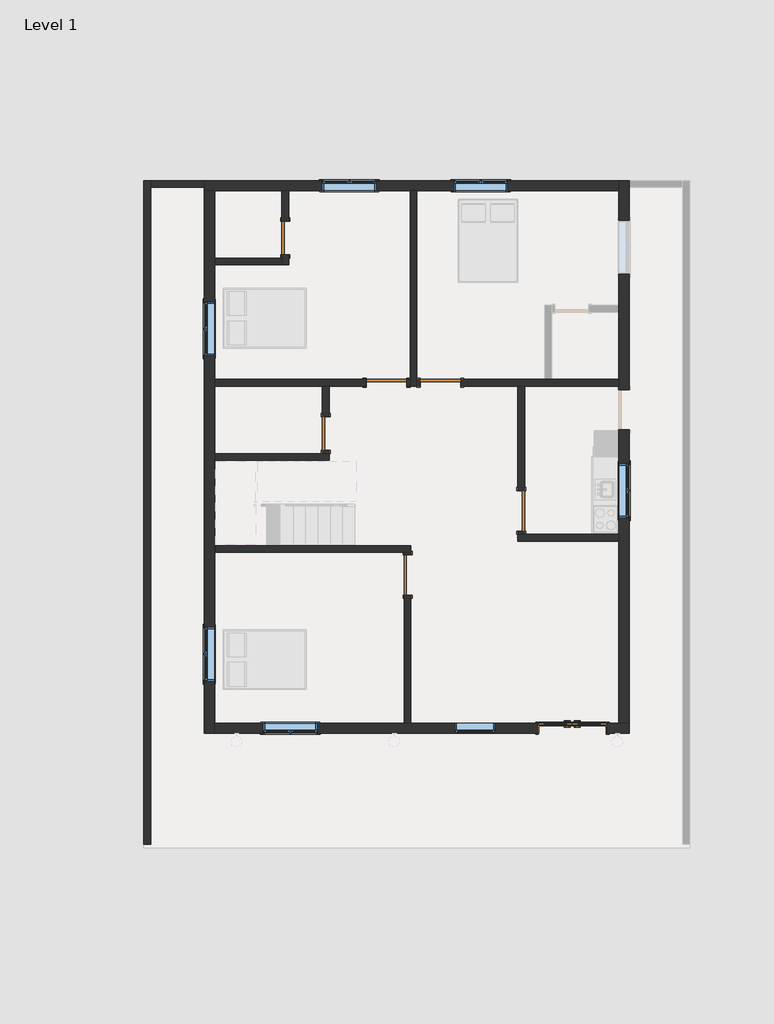
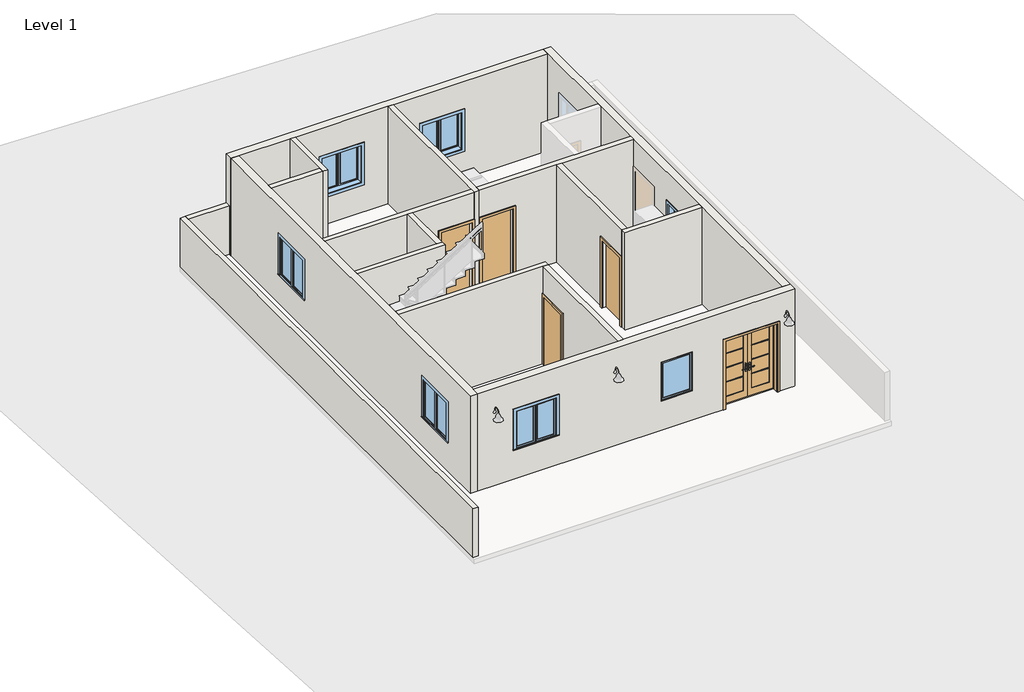
# One storey, part 1 of 2: 17 walls, 7 doors, 7 windows.
"""IFC4 building model written with IfcOpenShell, lengths in millimetres."""

from ifc_helpers import new_model, si_unit, frame, origin, origin_with_axes, place, context, project, spatial, polyline, outline, extrude, faceted_brep, transform, mapped, element, save
from components import door_014e9f54, single_flush_2_5_e2b13fe9, door_16372e1c, door_686f89d2, window_8af0dca1, window_c1f32544

model = new_model("IFC4")

# Units and contexts
model_context = context("Model", 3, world=origin())
ifc_project = project(units=[si_unit("LENGTHUNIT", "METRE", prefix="MILLI")], contexts=[model_context])

# Site, building, storey
site = spatial("IfcSite", under=ifc_project)
building = spatial("IfcBuilding", under=site)
storey = spatial("IfcBuildingStorey", under=building, Name="Level 1", Elevation=0.0)

# Doors
placement = place(None, origin())
door_shape = door_014e9f54(model_context)
element("IfcDoor", 1, ObjectType="Door-Exterior-Double-Full Glass-Wood_Clad : 60\" x 84\"", at=placement, inside=storey, context=model_context, shape_type="MappedRepresentation", body=[
    mapped(door_shape, transform((605.0352982, -4712.4924812, 0.0), x_axis=(1.0, 0.0, 0.0), y_axis=(0.0, 1.0, 0.0), z_axis=(0.0, 0.0, 1.0))),
])
single_flush_2_5_shape = single_flush_2_5_e2b13fe9(model_context)
element("IfcDoor", 2, ObjectType="Single-Flush : 2.5'", at=placement, inside=storey, context=model_context, shape_type="MappedRepresentation", body=[
    mapped(single_flush_2_5_shape, transform((-5884.6647018, 6371.4325188, 0.0), x_axis=(0.0, -1.0, 0.0), y_axis=(1.0, 0.0, 0.0), z_axis=(0.0, 0.0, 1.0))),
])
element("IfcDoor", 3, ObjectType="Single-Flush : 2.5'", at=placement, inside=storey, context=model_context, shape_type="MappedRepresentation", body=[
    mapped(single_flush_2_5_shape, transform((-4970.2647018, 1951.8325188, 0.0), x_axis=(0.0, -1.0, 0.0), y_axis=(1.0, 0.0, 0.0), z_axis=(0.0, 0.0, 1.0))),
])
door_2_shape = door_16372e1c(model_context)
element("IfcDoor", 4, ObjectType="Single-Flush : 36\" x 84\"", at=placement, inside=storey, context=model_context, shape_type="MappedRepresentation", body=[
    mapped(door_2_shape, transform((-3119.9591614, -1248.0450563, 0.0), x_axis=(0.0, 1.0, 0.0), y_axis=(-1.0, 0.0, 0.0), z_axis=(0.0, 0.0, 1.0))),
])
element("IfcDoor", 5, ObjectType="Single-Flush : 36\" x 84\"", at=placement, inside=storey, context=model_context, shape_type="MappedRepresentation", body=[
    mapped(door_2_shape, transform((-3598.6647018, 3094.8325188, 0.0), x_axis=(1.0, 0.0, 0.0), y_axis=(0.0, 1.0, 0.0), z_axis=(0.0, 0.0, 1.0))),
])
element("IfcDoor", 6, ObjectType="Single-Flush : 36\" x 84\"", at=placement, inside=storey, context=model_context, shape_type="MappedRepresentation", body=[
    mapped(door_2_shape, transform((-550.6647018, 199.2325188, 0.0), x_axis=(0.0, -1.0, 0.0), y_axis=(1.0, 0.0, 0.0), z_axis=(0.0, 0.0, 1.0))),
])
door_3_shape = door_686f89d2(model_context)
element("IfcDoor", 7, ObjectType="Single-Flush : 36\" x 84\"", at=placement, inside=storey, context=model_context, shape_type="MappedRepresentation", body=[
    mapped(door_3_shape, transform((-2379.4647018, 3094.8325188, 0.0), x_axis=(-1.0, 0.0, 0.0), y_axis=(0.0, -1.0, 0.0), z_axis=(0.0, 0.0, 1.0))),
])

# Walls
element("IfcWall", 8, ObjectType="6\"", at=placement, inside=storey, context=model_context, shape_type="Brep", body=[
    faceted_brep([(-8932.6647018, -7344.5674812, 0.0), (-8932.6647018, 7514.4325188, 0.0), (-8932.6647018, 7666.8325188, 0.0), (-8932.6647018, 7666.8325188, 1524.0), (-8932.6647018, 7514.4325188, 1524.0), (-8932.6647018, -7344.5674812, 1524.0), (-9085.0647018, -7344.5674812, 0.0), (-9085.0647018, -7344.5674812, 1524.0), (-9085.0647018, 7666.8325188, 1524.0), (-9085.0647018, 7666.8325188, 0.0)], [[[0, 1, 2, 3, 4, 5]], [[6, 7, 8, 9]], [[2, 1, 0, 6, 9]], [[5, 4, 3, 8, 7]], [[0, 5, 7, 6]], [[3, 2, 9, 8]]]),
])
element("IfcWall", 9, ObjectType="6\"", at=placement, inside=storey, context=model_context, shape_type="Brep", body=[
    faceted_brep([(-3065.2647018, 7438.2325188, 0.0), (-3065.2647018, 3171.0325188, 0.0), (-3065.2647018, 3018.6325188, 0.0), (-3065.2647018, 3018.6325188, 3048.0), (-3065.2647018, 3171.0325188, 3048.0), (-3065.2647018, 7438.2325188, 3048.0), (-2912.8647018, 7438.2325188, 0.0), (-2912.8647018, 7438.2325188, 3048.0), (-2912.8647018, 3171.0325188, 3048.0), (-2912.8647018, 3018.6325188, 3048.0), (-2912.8647018, 3018.6325188, 0.0), (-2912.8647018, 3171.0325188, 0.0)], [[[0, 1, 2, 3, 4, 5]], [[6, 7, 8, 9, 10, 11]], [[2, 1, 0, 6, 11, 10]], [[5, 4, 3, 9, 8, 7]], [[0, 5, 7, 6]], [[3, 2, 10, 9]]]),
])
element("IfcWall", 10, ObjectType="6\"", at=placement, inside=storey, context=model_context, shape_type="Brep", body=[
    faceted_brep([(-3065.2647018, 3171.0325188, 0.0), (-3141.4647018, 3171.0325188, 0.0), (-3141.4647018, 3171.0325188, 2133.6), (-4055.8647018, 3171.0325188, 2133.6), (-4055.8647018, 3171.0325188, 0.0), (-7484.8647018, 3171.0325188, 0.0), (-7484.8647018, 3171.0325188, 3048.0), (-3065.2647018, 3171.0325188, 3048.0), (-3141.4647018, 3018.6325188, 2133.6), (-3141.4647018, 3018.6325188, 0.0), (-3065.2647018, 3018.6325188, 0.0), (-3065.2647018, 3018.6325188, 3048.0), (-4894.0647018, 3018.6325188, 3048.0), (-5046.4647018, 3018.6325188, 3048.0), (-7484.8647018, 3018.6325188, 3048.0), (-7484.8647018, 3018.6325188, 0.0), (-5046.4647018, 3018.6325188, 0.0), (-4894.0647018, 3018.6325188, 0.0), (-4055.8647018, 3018.6325188, 0.0), (-4055.8647018, 3018.6325188, 2133.6)], [[[0, 1, 2, 3, 4, 5, 6, 7]], [[8, 9, 10, 11, 12, 13, 14, 15, 16, 17, 18, 19]], [[10, 9, 1, 0]], [[18, 17, 16, 15, 5, 4]], [[7, 6, 14, 13, 12, 11]], [[0, 7, 11, 10]], [[6, 5, 15, 14]], [[2, 1, 9, 8]], [[3, 2, 8, 19]], [[4, 3, 19, 18]]]),
])
element("IfcWall", 11, ObjectType="6\"", at=placement, inside=storey, context=model_context, shape_type="Brep", body=[
    faceted_brep([(-2912.8647018, 3018.6325188, 0.0), (-2836.6647018, 3018.6325188, 0.0), (-2836.6647018, 3018.6325188, 2133.6), (-1922.2647018, 3018.6325188, 2133.6), (-1922.2647018, 3018.6325188, 0.0), (-626.8647018, 3018.6325188, 0.0), (-474.4647018, 3018.6325188, 0.0), (1659.1352982, 3018.6325188, 0.0), (1659.1352982, 3018.6325188, 3048.0), (-474.4647018, 3018.6325188, 3048.0), (-626.8647018, 3018.6325188, 3048.0), (-2912.8647018, 3018.6325188, 3048.0), (-2836.6647018, 3171.0325188, 2133.6), (-2836.6647018, 3171.0325188, 0.0), (-2912.8647018, 3171.0325188, 0.0), (-2912.8647018, 3171.0325188, 3048.0), (-17.2647018, 3171.0325188, 3048.0), (135.1352982, 3171.0325188, 3048.0), (1659.1352982, 3171.0325188, 3048.0), (1659.1352982, 3171.0325188, 0.0), (135.1352982, 3171.0325188, 0.0), (-17.2647018, 3171.0325188, 0.0), (-1922.2647018, 3171.0325188, 0.0), (-1922.2647018, 3171.0325188, 2133.6)], [[[0, 1, 2, 3, 4, 5, 6, 7, 8, 9, 10, 11]], [[12, 13, 14, 15, 16, 17, 18, 19, 20, 21, 22, 23]], [[14, 13, 1, 0]], [[22, 21, 20, 19, 7, 6, 5, 4]], [[11, 10, 9, 8, 18, 17, 16, 15]], [[0, 11, 15, 14]], [[8, 7, 19, 18]], [[2, 1, 13, 12]], [[3, 2, 12, 23]], [[4, 3, 23, 22]]]),
])
element("IfcWall", 12, ObjectType="6\"", at=placement, inside=storey, context=model_context, shape_type="Brep", body=[
    faceted_brep([(-5960.8647018, 5990.4325188, 2133.6), (-5960.8647018, 5990.4325188, 0.0), (-5960.8647018, 5914.2325188, 0.0), (-5960.8647018, 5761.8325188, 0.0), (-5960.8647018, 5761.8325188, 3048.0), (-5960.8647018, 5914.2325188, 3048.0), (-5960.8647018, 7438.2325188, 3048.0), (-5960.8647018, 7438.2325188, 0.0), (-5960.8647018, 6752.4325188, 0.0), (-5960.8647018, 6752.4325188, 2133.6), (-5808.4647018, 5761.8325188, 0.0), (-5808.4647018, 5990.4325188, 0.0), (-5808.4647018, 5990.4325188, 2133.6), (-5808.4647018, 6752.4325188, 2133.6), (-5808.4647018, 6752.4325188, 0.0), (-5808.4647018, 7438.2325188, 0.0), (-5808.4647018, 7438.2325188, 3048.0), (-5808.4647018, 5761.8325188, 3048.0)], [[[0, 1, 2, 3, 4, 5, 6, 7, 8, 9]], [[10, 11, 12, 13, 14, 15, 16, 17]], [[8, 7, 15, 14]], [[3, 2, 1, 11, 10]], [[6, 5, 4, 17, 16]], [[7, 6, 16, 15]], [[4, 3, 10, 17]], [[12, 11, 1, 0]], [[13, 12, 0, 9]], [[14, 13, 9, 8]]]),
])
element("IfcWall", 13, ObjectType="6\"", at=placement, inside=storey, context=model_context, shape_type="SweptSolid", body=[
    extrude(outline(polyline([(-7484.8647018, 5914.2325188), (-5960.8647018, 5914.2325188), (-5960.8647018, 5761.8325188), (-7484.8647018, 5761.8325188), (-7484.8647018, 5914.2325188)])), origin_with_axes(), (0.0, 0.0, 1.0), 3048.0),
])
element("IfcWall", 14, ObjectType="6\"", at=placement, inside=storey, context=model_context, shape_type="Brep", body=[
    faceted_brep([(-7484.8647018, 1342.2325188, 0.0), (-4894.0647018, 1342.2325188, 0.0), (-4894.0647018, 1342.2325188, 3048.0), (-7484.8647018, 1342.2325188, 3048.0), (-7484.8647018, 1494.6325188, 0.0), (-7484.8647018, 1494.6325188, 3048.0), (-5046.4647018, 1494.6325188, 3048.0), (-4894.0647018, 1494.6325188, 3048.0), (-4894.0647018, 1494.6325188, 0.0), (-5046.4647018, 1494.6325188, 0.0)], [[[0, 1, 2, 3]], [[4, 5, 6, 7, 8, 9]], [[1, 0, 4, 9, 8]], [[3, 2, 7, 6, 5]], [[0, 3, 5, 4]], [[2, 1, 8, 7]]]),
])
element("IfcWall", 15, ObjectType="6\"", at=placement, inside=storey, context=model_context, shape_type="SweptSolid", body=[
    extrude(outline(polyline([(1570.8325188, 2133.6), (1570.8325188, 0.0), (1494.6325188, 0.0), (1494.6325188, 3048.0), (3018.6325188, 3048.0), (3018.6325188, 0.0), (2332.8325188, 0.0), (2332.8325188, 2133.6), (1570.8325188, 2133.6)])), frame((-5046.4647018, 0.0, 0.0), z_axis=(1.0, 0.0, 0.0), x_axis=(0.0, 1.0, 0.0)), (0.0, 0.0, 1.0), 152.4),
])
element("IfcWall", 16, ObjectType="6\"", at=placement, inside=storey, context=model_context, shape_type="SweptSolid", body=[
    extrude(outline(polyline([(-8932.6647018, 7666.8325188), (-7713.4647018, 7666.8325188), (-7713.4647018, 7514.4325188), (-8932.6647018, 7514.4325188), (-8932.6647018, 7666.8325188)])), origin_with_axes(), (0.0, 0.0, 1.0), 1524.0),
])
element("IfcWall", 17, ObjectType="6\"", at=placement, inside=storey, context=model_context, shape_type="Brep", body=[
    faceted_brep([(1659.1352982, -334.1674812, 0.0), (-474.4647018, -334.1674812, 0.0), (-626.8647018, -334.1674812, 0.0), (-626.8647018, -334.1674812, 3048.0), (-474.4647018, -334.1674812, 3048.0), (1659.1352982, -334.1674812, 3048.0), (1659.1352982, -486.5674812, 0.0), (1659.1352982, -486.5674812, 3048.0), (-626.8647018, -486.5674812, 3048.0), (-626.8647018, -486.5674812, 0.0)], [[[0, 1, 2, 3, 4, 5]], [[6, 7, 8, 9]], [[2, 1, 0, 6, 9]], [[5, 4, 3, 8, 7]], [[0, 5, 7, 6]], [[3, 2, 9, 8]]]),
])
element("IfcWall", 18, ObjectType="6\"", at=placement, inside=storey, context=model_context, shape_type="SweptSolid", body=[
    extrude(outline(polyline([(-257.9674812, 2133.6), (-257.9674812, 0.0), (-334.1674812, 0.0), (-334.1674812, 3048.0), (3018.6325188, 3048.0), (3018.6325188, 0.0), (656.4325188, 0.0), (656.4325188, 2133.6), (-257.9674812, 2133.6)])), frame((-626.8647018, 0.0, 0.0), z_axis=(1.0, 0.0, 0.0), x_axis=(0.0, 1.0, 0.0)), (0.0, 0.0, 1.0), 152.4),
])
element("IfcWall", 19, ObjectType="6\"", at=placement, inside=storey, context=model_context, shape_type="Brep", body=[
    faceted_brep([(-7463.3591614, -740.0450563, 0.0), (-3196.1591614, -740.0450563, 0.0), (-3043.7591614, -740.0450563, 0.0), (-3043.7591614, -740.0450563, 3048.0), (-3196.1591614, -740.0450563, 3048.0), (-7463.3591614, -740.0450563, 3048.0), (-7463.3591614, -587.6450563, 0.0), (-7463.3591614, -587.6450563, 3048.0), (-3043.7591614, -587.6450563, 3048.0), (-3043.7591614, -587.6450563, 0.0)], [[[0, 1, 2, 3, 4, 5]], [[6, 7, 8, 9]], [[2, 1, 0, 6, 9]], [[5, 4, 3, 8, 7]], [[0, 5, 7, 6]], [[3, 2, 9, 8]]]),
])
element("IfcWall", 20, ObjectType="6\"", at=placement, inside=storey, context=model_context, shape_type="SweptSolid", body=[
    extrude(outline(polyline([(-740.0450563, 0.0), (-790.8450563, 0.0), (-790.8450563, 2133.6), (-1705.2450563, 2133.6), (-1705.2450563, 0.0), (-4601.3674812, 0.0), (-4601.3674812, 3048.0), (-740.0450563, 3048.0), (-740.0450563, 0.0)])), frame((-3196.1591614, 0.0, 0.0), z_axis=(1.0, 0.0, 0.0), x_axis=(0.0, 1.0, 0.0)), (0.0, 0.0, 1.0), 152.4),
])
element("IfcWall", 21, ObjectType="9\"", at=placement, inside=storey, context=model_context, shape_type="Brep", body=[
    faceted_brep([(-7713.4647018, 7438.2325188, 3048.0), (-7713.4647018, 7438.2325188, 0.0), (-7713.4647018, -4829.9674812, 0.0), (-7713.4647018, -4829.9674812, 3048.0), (-7713.4647018, -2429.6674812, 2133.6), (-7713.4647018, -3648.8674812, 2133.6), (-7713.4647018, -3648.8674812, 914.4), (-7713.4647018, -2429.6674812, 914.4), (-7713.4647018, 4923.6325188, 2133.6), (-7713.4647018, 3704.4325188, 2133.6), (-7713.4647018, 3704.4325188, 914.4), (-7713.4647018, 4923.6325188, 914.4), (-7484.8647018, 7438.2325188, 0.0), (-7484.8647018, 7438.2325188, 3048.0), (-7484.8647018, 5914.2325188, 3048.0), (-7484.8647018, 5761.8325188, 3048.0), (-7484.8647018, 3171.0325188, 3048.0), (-7484.8647018, 3018.6325188, 3048.0), (-7484.8647018, 1494.6325188, 3048.0), (-7484.8647018, 1342.2325188, 3048.0), (-7484.8647018, -4601.3674812, 3048.0), (-7484.8647018, -4829.9674812, 3048.0), (-7484.8647018, -4829.9674812, 0.0), (-7484.8647018, -4601.3674812, 0.0), (-7484.8647018, 1342.2325188, 0.0), (-7484.8647018, 1494.6325188, 0.0), (-7484.8647018, 3018.6325188, 0.0), (-7484.8647018, 3171.0325188, 0.0), (-7484.8647018, 5761.8325188, 0.0), (-7484.8647018, 5914.2325188, 0.0), (-7484.8647018, -2429.6674812, 2133.6), (-7484.8647018, -2429.6674812, 914.4), (-7484.8647018, -3648.8674812, 914.4), (-7484.8647018, -3648.8674812, 2133.6), (-7484.8647018, 4923.6325188, 2133.6), (-7484.8647018, 4923.6325188, 914.4), (-7484.8647018, 3704.4325188, 914.4), (-7484.8647018, 3704.4325188, 2133.6)], [[[0, 1, 2, 3], [4, 5, 6, 7], [8, 9, 10, 11]], [[12, 13, 14, 15, 16, 17, 18, 19, 20, 21, 22, 23, 24, 25, 26, 27, 28, 29], [30, 31, 32, 33], [34, 35, 36, 37]], [[2, 1, 12, 29, 28, 27, 26, 25, 24, 23, 22]], [[0, 3, 21, 20, 19, 18, 17, 16, 15, 14, 13]], [[3, 2, 22, 21]], [[0, 13, 12, 1]], [[31, 30, 4, 7]], [[32, 31, 7, 6]], [[33, 32, 6, 5]], [[30, 33, 5, 4]], [[35, 34, 8, 11]], [[36, 35, 11, 10]], [[37, 36, 10, 9]], [[34, 37, 9, 8]]]),
])
element("IfcWall", 22, ObjectType="9\"", at=placement, inside=storey, context=model_context, shape_type="Brep", body=[
    faceted_brep([(1887.7352982, -4829.9674812, 3048.0), (-7484.8647018, -4829.9674812, 3048.0), (-7484.8647018, -4829.9674812, 0.0), (-182.3647018, -4829.9674812, 0.0), (-182.3647018, -4829.9674812, 2159.0), (1392.4352982, -4829.9674812, 2159.0), (1392.4352982, -4829.9674812, 0.0), (1887.7352982, -4829.9674812, 0.0), (-2053.1591614, -4829.9674812, 2133.6), (-1138.7591614, -4829.9674812, 2133.6), (-1138.7591614, -4829.9674812, 914.4), (-2053.1591614, -4829.9674812, 914.4), (-6379.9647018, -4829.9674812, 2133.6), (-5160.7647018, -4829.9674812, 2133.6), (-5160.7647018, -4829.9674812, 914.4), (-6379.9647018, -4829.9674812, 914.4), (-7484.8647018, -4601.3674812, 3048.0), (-3196.1591614, -4601.3674812, 3048.0), (-3043.7591614, -4601.3674812, 3048.0), (1659.1352982, -4601.3674812, 3048.0), (1887.7352982, -4601.3674812, 3048.0), (1887.7352982, -4601.3674812, 0.0), (1659.1352982, -4601.3674812, 0.0), (1392.4352982, -4601.3674812, 0.0), (1392.4352982, -4601.3674812, 2159.0), (-182.3647018, -4601.3674812, 2159.0), (-182.3647018, -4601.3674812, 0.0), (-3043.7591614, -4601.3674812, 0.0), (-3196.1591614, -4601.3674812, 0.0), (-7484.8647018, -4601.3674812, 0.0), (-2053.1591614, -4601.3674812, 2133.6), (-2053.1591614, -4601.3674812, 914.4), (-1138.7591614, -4601.3674812, 914.4), (-1138.7591614, -4601.3674812, 2133.6), (-6379.9647018, -4601.3674812, 2133.6), (-6379.9647018, -4601.3674812, 914.4), (-5160.7647018, -4601.3674812, 914.4), (-5160.7647018, -4601.3674812, 2133.6)], [[[0, 1, 2, 3, 4, 5, 6, 7], [8, 9, 10, 11], [12, 13, 14, 15]], [[16, 17, 18, 19, 20, 21, 22, 23, 24, 25, 26, 27, 28, 29], [30, 31, 32, 33], [34, 35, 36, 37]], [[2, 29, 28, 27, 26, 3]], [[21, 7, 6, 23, 22]], [[1, 0, 20, 19, 18, 17, 16]], [[2, 1, 16, 29]], [[0, 7, 21, 20]], [[5, 24, 23, 6]], [[24, 5, 4, 25]], [[25, 4, 3, 26]], [[31, 30, 8, 11]], [[32, 31, 11, 10]], [[33, 32, 10, 9]], [[30, 33, 9, 8]], [[35, 34, 12, 15]], [[36, 35, 15, 14]], [[37, 36, 14, 13]], [[34, 37, 13, 12]]]),
])
element("IfcWall", 23, ObjectType="9\"", at=placement, inside=storey, context=model_context, shape_type="Brep", body=[
    faceted_brep([(1887.7352982, 2942.4325188, 2133.6), (1887.7352982, 2942.4325188, 0.0), (1887.7352982, 7514.4325188, 0.0), (1887.7352982, 7666.8325188, 0.0), (1887.7352982, 7666.8325188, 1524.0), (1887.7352982, 7666.8325188, 3048.0), (1887.7352982, -4601.3674812, 3048.0), (1887.7352982, -4601.3674812, 0.0), (1887.7352982, 2028.0325188, 0.0), (1887.7352982, 2028.0325188, 2133.6), (1887.7352982, 5552.2825188, 2133.6), (1887.7352982, 6771.4825188, 2133.6), (1887.7352982, 6771.4825188, 914.4), (1887.7352982, 5552.2825188, 914.4), (1887.7352982, 46.8325188, 2133.6), (1887.7352982, 1266.0325188, 2133.6), (1887.7352982, 1266.0325188, 914.4), (1887.7352982, 46.8325188, 914.4), (1659.1352982, 7666.8325188, 0.0), (1659.1352982, 7438.2325188, 0.0), (1659.1352982, 4847.4325188, 0.0), (1659.1352982, 4695.0325188, 0.0), (1659.1352982, 3171.0325188, 0.0), (1659.1352982, 3018.6325188, 0.0), (1659.1352982, 2942.4325188, 0.0), (1659.1352982, 2942.4325188, 2133.6), (1659.1352982, 2028.0325188, 2133.6), (1659.1352982, 2028.0325188, 0.0), (1659.1352982, -334.1674812, 0.0), (1659.1352982, -486.5674812, 0.0), (1659.1352982, -4601.3674812, 0.0), (1659.1352982, -4601.3674812, 3048.0), (1659.1352982, -486.5674812, 3048.0), (1659.1352982, -334.1674812, 3048.0), (1659.1352982, 3018.6325188, 3048.0), (1659.1352982, 3171.0325188, 3048.0), (1659.1352982, 4695.0325188, 3048.0), (1659.1352982, 4847.4325188, 3048.0), (1659.1352982, 7438.2325188, 3048.0), (1659.1352982, 7666.8325188, 3048.0), (1659.1352982, 5552.2825188, 2133.6), (1659.1352982, 5552.2825188, 914.4), (1659.1352982, 6771.4825188, 914.4), (1659.1352982, 6771.4825188, 2133.6), (1659.1352982, 46.8325188, 2133.6), (1659.1352982, 46.8325188, 914.4), (1659.1352982, 1266.0325188, 914.4), (1659.1352982, 1266.0325188, 2133.6)], [[[0, 1, 2, 3, 4, 5, 6, 7, 8, 9], [10, 11, 12, 13], [14, 15, 16, 17]], [[18, 19, 20, 21, 22, 23, 24, 25, 26, 27, 28, 29, 30, 31, 32, 33, 34, 35, 36, 37, 38, 39], [40, 41, 42, 43], [44, 45, 46, 47]], [[8, 7, 30, 29, 28, 27]], [[3, 2, 1, 24, 23, 22, 21, 20, 19, 18]], [[6, 5, 39, 38, 37, 36, 35, 34, 33, 32, 31]], [[7, 6, 31, 30]], [[3, 18, 39, 5, 4]], [[25, 24, 1, 0]], [[26, 25, 0, 9]], [[27, 26, 9, 8]], [[41, 40, 10, 13]], [[42, 41, 13, 12]], [[43, 42, 12, 11]], [[40, 43, 11, 10]], [[45, 44, 14, 17]], [[46, 45, 17, 16]], [[47, 46, 16, 15]], [[44, 47, 15, 14]]]),
])
element("IfcWall", 24, ObjectType="9\"", at=placement, inside=storey, context=model_context, shape_type="Brep", body=[
    faceted_brep([(-7713.4647018, 7438.2325188, 3048.0), (-7713.4647018, 7438.2325188, 0.0), (-7484.8647018, 7438.2325188, 0.0), (-5960.8647018, 7438.2325188, 0.0), (-5808.4647018, 7438.2325188, 0.0), (-3065.2647018, 7438.2325188, 0.0), (-2912.8647018, 7438.2325188, 0.0), (1659.1352982, 7438.2325188, 0.0), (1659.1352982, 7438.2325188, 3048.0), (-2912.8647018, 7438.2325188, 3048.0), (-3065.2647018, 7438.2325188, 3048.0), (-5808.4647018, 7438.2325188, 3048.0), (-5960.8647018, 7438.2325188, 3048.0), (-7484.8647018, 7438.2325188, 3048.0), (-3827.2647018, 7438.2325188, 2133.6), (-3827.2647018, 7438.2325188, 914.4), (-5046.4647018, 7438.2325188, 914.4), (-5046.4647018, 7438.2325188, 2133.6), (-855.4647018, 7438.2325188, 2133.6), (-855.4647018, 7438.2325188, 914.4), (-2074.6647018, 7438.2325188, 914.4), (-2074.6647018, 7438.2325188, 2133.6), (-7713.4647018, 7666.8325188, 0.0), (-7713.4647018, 7666.8325188, 3048.0), (1659.1352982, 7666.8325188, 3048.0), (1659.1352982, 7666.8325188, 0.0), (-3827.2647018, 7666.8325188, 2133.6), (-5046.4647018, 7666.8325188, 2133.6), (-5046.4647018, 7666.8325188, 914.4), (-3827.2647018, 7666.8325188, 914.4), (-855.4647018, 7666.8325188, 2133.6), (-2074.6647018, 7666.8325188, 2133.6), (-2074.6647018, 7666.8325188, 914.4), (-855.4647018, 7666.8325188, 914.4), (-7713.4647018, 7514.4325188, 0.0)], [[[0, 1, 2, 3, 4, 5, 6, 7, 8, 9, 10, 11, 12, 13], [14, 15, 16, 17], [18, 19, 20, 21]], [[22, 23, 24, 25], [26, 27, 28, 29], [30, 31, 32, 33]], [[7, 6, 5, 4, 3, 2, 1, 34, 22, 25]], [[0, 13, 12, 11, 10, 9, 8, 24, 23]], [[7, 25, 24, 8]], [[0, 23, 22, 34, 1]], [[15, 14, 26, 29]], [[16, 15, 29, 28]], [[17, 16, 28, 27]], [[14, 17, 27, 26]], [[19, 18, 30, 33]], [[20, 19, 33, 32]], [[21, 20, 32, 31]], [[18, 21, 31, 30]]]),
])

# Windows
window_shape = window_8af0dca1(model_context)
element("IfcWindow", 25, ObjectType="Casement Dbl with Trim : 48\" x 48\"", at=placement, inside=storey, context=model_context, shape_type="MappedRepresentation", body=[
    mapped(window_shape, transform((-5770.3647018, -4696.6174812, 152.4), x_axis=(-1.0, 0.0, 0.0), y_axis=(0.0, -1.0, 0.0), z_axis=(0.0, 0.0, 1.0))),
])
element("IfcWindow", 26, ObjectType="Casement Dbl with Trim : 48\" x 48\"", at=placement, inside=storey, context=model_context, shape_type="MappedRepresentation", body=[
    mapped(window_shape, transform((-7580.1147018, -3039.2674812, 152.4), x_axis=(0.0, 1.0, 0.0), y_axis=(-1.0, 0.0, 0.0), z_axis=(0.0, 0.0, 1.0))),
])
element("IfcWindow", 27, ObjectType="Casement Dbl with Trim : 48\" x 48\"", at=placement, inside=storey, context=model_context, shape_type="MappedRepresentation", body=[
    mapped(window_shape, transform((-7580.1147018, 4314.0325188, 152.4), x_axis=(0.0, 1.0, 0.0), y_axis=(-1.0, 0.0, 0.0), z_axis=(0.0, 0.0, 1.0))),
])
element("IfcWindow", 28, ObjectType="Casement Dbl with Trim : 48\" x 48\"", at=placement, inside=storey, context=model_context, shape_type="MappedRepresentation", body=[
    mapped(window_shape, transform((-4436.8647018, 7533.4825188, 152.4), x_axis=(1.0, 0.0, 0.0), y_axis=(0.0, 1.0, 0.0), z_axis=(0.0, 0.0, 1.0))),
])
element("IfcWindow", 29, ObjectType="Casement Dbl with Trim : 48\" x 48\"", at=placement, inside=storey, context=model_context, shape_type="MappedRepresentation", body=[
    mapped(window_shape, transform((-1465.0647018, 7533.4825188, 152.4), x_axis=(1.0, 0.0, 0.0), y_axis=(0.0, 1.0, 0.0), z_axis=(0.0, 0.0, 1.0))),
])
element("IfcWindow", 30, ObjectType="Casement Dbl with Trim : 48\" x 48\"", at=placement, inside=storey, context=model_context, shape_type="MappedRepresentation", body=[
    mapped(window_shape, transform((1754.3852982, 656.4325188, 152.4), x_axis=(0.0, -1.0, 0.0), y_axis=(1.0, 0.0, 0.0), z_axis=(0.0, 0.0, 1.0))),
])
window_2_shape = window_c1f32544(model_context)
element("IfcWindow", 31, ObjectType="Fixed : 36\" x 48\"", at=placement, inside=storey, context=model_context, shape_type="MappedRepresentation", body=[
    mapped(window_2_shape, transform((-1634.0591614, -4715.6674812, 0.0), x_axis=(-1.0, 0.0, 0.0), y_axis=(0.0, -1.0, 0.0), z_axis=(0.0, 0.0, 1.0))),
])

save(model, "model.ifc")

# Revit data of these elements
# Type "Door-Exterior-Double-Full Glass-Wood_Clad : 60\" x 84\""
#   Type Mark = "9"
#   Assembly Code = "B2030100"
#   Analytic Construction = "French door, wood frame with double glass"
#   Top Rail = 0' - 4 11/16"
#   Threshold Offset [instance default] = 0' - 0 1/2"
#   Thickness = 0' - 1 3/8"
#   Thermal Resistance (R) = 1.9158 (h·ft²·°F)/BTU
#   Swing Angle [instance default] = 90.00°
#   Stiles = 0' - 4 3/4"
#   Rough Width = 5' - 2"
#   Rough Height = 7' - 1"
#   Panel Width = 2' - 6"
#   Door Offset [instance default] = 0' - 0"
#   Height = 7' - 0"
#   Width = 5' - 0"
#   Heat Transfer Coefficient (U) = 0.5220 BTU/(h·ft²·°F)
#   Bottom Rail = 0' - 9 1/8"
#   Exterior Trim [instance default] = yes
#   Threshold [instance default] = yes
#   Show Grill [instance default] = yes
#   Function = 1
#   Trim Material = Cherry
#   Threshold Material = Cherry
#   Panel Material = Cherry
#   Glazing = Glass
#   Frame Material = Cherry
#   Door Handle Material = Aluminum
#   Visual Light Transmittance = 0
#   Solar Heat Gain Coefficient = 0
#   Wall Closure = (empty or 0)
#   Construction Type = (empty or 0)
# Type "Single-Flush : 2.5'"
#   Type Mark = "8"
#   Construction Type Id = "MDOOR"
#   Assembly Code = "C1020"
#   Analytic Construction = "Metal"
#   Thickness = 0' - 2"
#   Heat Transfer Coefficient (U) = 0.651978 BTU/(h·ft²·°F)
#   Height = 7' - 0"
#   Trim Projection Ext = 0' - 1"
#   Trim Projection Int = 0' - 1"
#   Trim Width = 0' - 3"
#   Width = 2' - 6"
#   Define Thermal Properties by = 1
#   Door Material = Door - Panel
#   Frame Material = Door - Frame
#   Visual Light Transmittance = 0
#   Solar Heat Gain Coefficient = 0
#   Function = (empty or 0)
#   Wall Closure = (empty or 0)
# Type "Single-Flush : 36\" x 84\""
#   Type Mark = "1"
#   Construction Type Id = "MDOOR"
#   Assembly Code = "C1020"
#   Analytic Construction = "Metal"
#   Thickness = 0' - 2"
#   Heat Transfer Coefficient (U) = 0.651978 BTU/(h·ft²·°F)
#   Height = 7' - 0"
#   Trim Projection Ext = 0' - 1"
#   Trim Projection Int = 0' - 1"
#   Trim Width = 0' - 3"
#   Width = 3' - 0"
#   Define Thermal Properties by = 1
#   Door Material = Door - Panel
#   Frame Material = Door - Frame
#   Visual Light Transmittance = 0
#   Solar Heat Gain Coefficient = 0
#   Function = (empty or 0)
#   Wall Closure = (empty or 0)
# Type "6\""
#   Assembly Code = "B2010"
#   Layers, outside or top first: 0' - 6" "inner wall" (function 1)
# Type "9\""
#   Assembly Code = "B2010"
#   Layers, outside or top first: 0' - 9" "ext wall" (function 1)
# Type "Casement Dbl with Trim : 48\" x 48\""
#   Type Mark = "10"
#   Construction Type Id = "GSP4R"
#   Assembly Code = "B2020100"
#   Analytic Construction = "1/8 in Pilkington single glazing"
#   Visual Light Transmittance = 0.9
#   Solar Heat Gain Coefficient = 0.78
#   Heat Transfer Coefficient (U) = 0.6496 BTU/(h·ft²·°F)
#   Height = 4' - 0"
#   Default Sill Height = 2' - 6"
#   Trim Projection - Ext. = 0' - 0 1/2"
#   Trim Projection - Int. = 0' - 0 3/4"
#   Trim Width - Exterior = 0' - 3 1/2"
#   Trim Width - Interior = 0' - 3 1/2"
#   Width = 4' - 0"
#   Window Inset = 0' - 0 3/4"
#   Define Thermal Properties by = 1
#   Glass Pane Material = Glass
#   Sash Material = Sash
#   Trim Exterior Material = Trim
#   Trim Interior Material = Trim
#   Wall Closure = (empty or 0)
# Type "Fixed : 36\" x 48\""
#   Type Mark = "1"
#   Construction Type Id = "GSP4R"
#   Assembly Code = "B2020100"
#   Analytic Construction = "1/8 in Pilkington single glazing"
#   Visual Light Transmittance = 0.9
#   Solar Heat Gain Coefficient = 0.78
#   Heat Transfer Coefficient (U) = 0.6496 BTU/(h·ft²·°F)
#   Height = 4' - 0"
#   Default Sill Height = 3' - 0"
#   Width = 3' - 0"
#   Window Inset = 0' - 0 3/4"
#   Define Thermal Properties by = 1
#   Glass Pane Material = Glass
#   Sash Material = Sash
#   Wall Closure = (empty or 0)
# Element 1 (IfcDoor, "Door-Exterior-Double-Full Glass-Wood_Clad : 60\" x 84\"")
#   Threshold Offset = 0' - 0 1/2"
#   Swing Angle = 90.00°
#   Door Offset = 0' - 0"
#   Threshold = yes
#   Show Grill = yes
#   Exterior Trim = yes
#   Phase Created = New Construction
#   Materials on its faces: "Cherry", "Aluminum", "Glass"
# Elements 2, 3 (IfcDoor, "Single-Flush : 2.5'")
#   Phase Created = New Construction
#   Materials on its faces: "Door - Frame", "Door - Panel"
# Elements 4, 5, 6, 7 (IfcDoor, "Single-Flush : 36\" x 84\"")
#   Phase Created = New Construction
#   Materials on its faces: "Door - Frame", "Door - Panel"
# Elements 8, 16 (IfcWall, "6\"")
#   Top Offset = 0' - 0"
#   Base Offset = 0' - 0"
#   Unconnected Height = 5' - 0"
#   wall height = 5' - 0"
#   Phase Created = New Construction
#   Base Constraint = Level 1
#   Materials on its faces: "inner wall"
# Elements 9, 10, 11, 12, 13, 14, 15, 17, 18, 19, 20 (IfcWall, "6\"")
#   Top Offset = 0' - 0"
#   Base Offset = 0' - 0"
#   Unconnected Height = 10' - 0"
#   wall height = 10' - 0"
#   Phase Created = New Construction
#   Base Constraint = Level 1
#   Materials on its faces: "inner wall"
# Elements 21, 22, 23, 24 (IfcWall, "9\"")
#   Top Offset = 0' - 0"
#   Base Offset = 0' - 0"
#   Unconnected Height = 10' - 0"
#   wall height = 10' - 0"
#   Phase Created = New Construction
#   Base Constraint = Level 1
#   Materials on its faces: "ext wall", "inner wall"
# Element 25 (IfcWindow, "Casement Dbl with Trim : 48\" x 48\"")
#   Mark = "2"
#   Phase Created = New Construction
#   Materials on its faces: "Sash", "Trim", "Glass"
# Element 26 (IfcWindow, "Casement Dbl with Trim : 48\" x 48\"")
#   Mark = "3"
#   Phase Created = New Construction
#   Materials on its faces: "Sash", "Trim", "Glass"
# Element 27 (IfcWindow, "Casement Dbl with Trim : 48\" x 48\"")
#   Mark = "4"
#   Phase Created = New Construction
#   Materials on its faces: "Sash", "Trim", "Glass"
# Element 28 (IfcWindow, "Casement Dbl with Trim : 48\" x 48\"")
#   Mark = "5"
#   Phase Created = New Construction
#   Materials on its faces: "Sash", "Trim", "Glass"
# Element 29 (IfcWindow, "Casement Dbl with Trim : 48\" x 48\"")
#   Mark = "6"
#   Phase Created = New Construction
#   Materials on its faces: "Sash", "Trim", "Glass"
# Element 30 (IfcWindow, "Casement Dbl with Trim : 48\" x 48\"")
#   Mark = "8"
#   Phase Created = New Construction
#   Materials on its faces: "Sash", "Trim", "Glass"
# Element 31 (IfcWindow, "Fixed : 36\" x 48\"")
#   Mark = "1"
#   Phase Created = New Construction
#   Materials on its faces: "Sash", "Glass"
# Materials
#   "Cherry": class "Wood", colour RGB 226 177 128, transparency 0, Description = "Prunus Serotina", Cost = 0
#   "Glass": class "Glass", colour RGB 0 128 192, transparency 0.75, Description = "Soda Lime Glass", Cost = 0
#   "Aluminum": class "Metal", colour RGB 247 247 247, transparency 0, Description = "Aluminum 6061", Cost = 0
#   "Door - Panel": class "Wood", colour RGB 210 159 95, transparency 0
#   "Door - Frame": colour RGB 118 70 51, transparency 0
#   "inner wall": class "Generic", colour RGB 230 213 172, transparency 0, Cost = 0
#   "ext wall": class "Generic", colour RGB 153 153 153, transparency 0, Cost = 0
#   "Sash": class "Wood", colour RGB 224 178 126, transparency 0
#   "Trim": class "Wood", colour RGB 224 178 126, transparency 0
